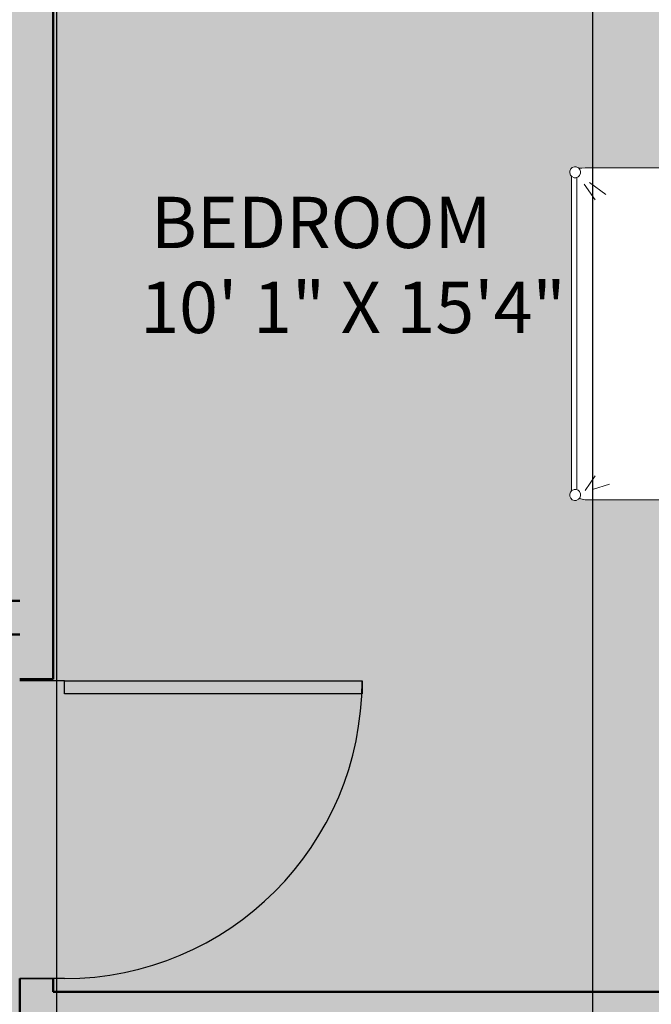
# Model space of a CAD drawing. Units: inches. Extents: x 528 to 2620, y -1066 to 798.
# Tile 32 of 41: x 1211 to 1296, y 524 to 656. Entities that reach past the tile are written whole.
import ezdxf

# ---------------------------------------------------------------- set-up
doc = ezdxf.new("R2010")
doc.units = ezdxf.units.IN
doc.header["$MEASUREMENT"] = 0
for name, color, linetype, lineweight in [('A-ANNO-DIMS', 2, 'Continuous', 18), ('A-AREA-IDEN', 7, 'Continuous', 18), ('A-Door', 2, 'Continuous', 25), ('A-FURN', 30, 'Continuous', 18), ('A-WALL', 7, 'Continuous', 50), ('A-WALL-PATT', 8, 'Continuous', 13)]:
    doc.layers.add(name, color=color, linetype=linetype, lineweight=lineweight)
doc.styles.get("Standard").update_dxf_attribs({"font": 'arial.ttf'})
doc.dimstyles.get("Standard").update_dxf_attribs({"dimtxt": 6, "dimasz": 2, "dimexe": 0.18, "dimexo": 0.0625, "dimgap": 0.09, "dimtad": 0, "dimtih": 1, "dimtoh": 1, "dimdec": 1, "dimzin": 0, "dimdsep": 46, "dimlunit": 3, "dimtxsty": 'Standard', "dimblk": 'ARCHTICK', "dimcen": 0.09, "dimadec": 0, "dimazin": 0, "dimtfac": 1, "dimtdec": 1, "dimtofl": 0, "dimtmove": 0, "dimatfit": 3, "dimfxl": 1, "dimtolj": 1, "dimtzin": 0, "dimarcsym": 0})

# ---------------------------------------------------------------- blocks, each defined once
blk = doc.blocks.new('*U4')
for p, q in [((0, 0), (0, -6)), ((40, 0), (40, -6))]:
    blk.add_line(p, q)
blk.add_lwpolyline([(0, 0), (0, 40), (1.75, 40), (1.75, 0)], close=True)
blk.add_arc((0, 0), 40, 0, 90)
blk = doc.blocks.new('d-bed-3')
at = {"color": 0, "linetype": 'ByBlock'}
for p, q in [((0, 0), (0, -0.5)), ((0.7, 0), (0, 0)), ((0.7, -0.5), (0.7, 0)), ((0.7817, -0.0054), (0.7857, 0.0078)), ((0.7817, -0.0054), (0.7857, 0.0078)), ((0.7857, 0.0078), (0.7968, 0.0166)), ((0.7857, 0.0078), (0.7968, 0.0166)), ((0.7968, 0.0166), (0.8078, 0.0211)), ((0.7968, 0.0166), (0.8078, 0.0211)), ((0.8078, 0.0211), (0.8209, 0.0211)), ((0.8078, 0.0211), (0.8209, 0.0211)), ((0.8209, 0.0211), (0.8349, 0.0144)), ((0.8209, 0.0211), (0.8349, 0.0144)), ((0.8349, 0.0144), (0.8409, 0.0078)), ((0.8349, 0.0144), (0.8429, 0.0056)), ((0.8389, 0.0078), (2.7305, 0.0078)), ((0.8409, 0.0078), (2.7305, 0.0078)), ((0.8429, 0.0056), (0.848, -0.0077)), ((2.7234, -0.0077), (2.7284, 0.0056)), ((2.7284, 0.0056), (2.7365, 0.0144)), ((2.7305, 0.0078), (2.7365, 0.0144)), ((2.7365, 0.0144), (2.7505, 0.0211)), ((2.7365, 0.0144), (2.7505, 0.0211)), ((2.7505, 0.0211), (2.7636, 0.0211)), ((2.7505, 0.0211), (2.7636, 0.0211)), ((2.7636, 0.0211), (2.7746, 0.0166)), ((2.7636, 0.0211), (2.7746, 0.0166)), ((2.7746, 0.0166), (2.7857, 0.0078)), ((2.7746, 0.0166), (2.7857, 0.0078)), ((2.7857, 0.0078), (2.7897, -0.0054)), ((2.7857, 0.0078), (2.7897, -0.0054)), ((2.8714, -0.5), (2.8714, 0)), ((2.8714, 0), (3.5714, 0)), ((3.5714, 0), (3.5714, -0.5)), ((0.05, -0.05), (0.05, -0.45)), ((0.65, -0.05), (0.05, -0.05)), ((0.35, -0.0576), (0.35, -0.4424)), ((0.65, -0.45), (0.65, -0.05)), ((0.7817, -0.0187), (0.7817, -0.0054)), ((0.7817, -0.0187), (0.7817, -0.0054)), ((0.7857, -0.0297), (0.7817, -0.0187)), ((0.7857, -0.0297), (0.7817, -0.0187)), ((0.7857, -2.0939), (0.7857, -0.0297)), ((0.7948, -0.0408), (0.7857, -0.0297)), ((0.7857, -0.032), (0.7857, -2.0939)), ((0.8058, -0.0452), (0.7948, -0.0408)), ((0.8188, -0.0452), (0.8058, -0.0452)), ((0.8319, -0.0408), (0.8188, -0.0452)), ((2.7525, -0.0452), (0.8188, -0.0452)), ((0.8409, -0.032), (0.8319, -0.0408)), ((0.848, -0.0209), (0.8409, -0.032)), ((0.848, -0.0077), (0.848, -0.0209)), ((2.7234, -0.0209), (2.7234, -0.0077)), ((2.7305, -0.032), (2.7234, -0.0209)), ((2.7395, -0.0408), (2.7305, -0.032)), ((2.7525, -0.0452), (2.7395, -0.0408)), ((2.7656, -0.0452), (2.7525, -0.0452)), ((2.7766, -0.0408), (2.7656, -0.0452)), ((2.7766, -0.0408), (2.7656, -0.0452)), ((2.7656, -0.0452), (2.7857, -0.0452)), ((2.7857, -0.0452), (2.7656, -0.0452)), ((2.7857, -0.0297), (2.7766, -0.0408)), ((2.7857, -0.0297), (2.7766, -0.0408)), ((2.7897, -0.0187), (2.7857, -0.0297)), ((2.7897, -0.0187), (2.7857, -0.0297)), ((2.7857, -2.0939), (2.7857, -0.0452)), ((2.7897, -0.0054), (2.7897, -0.0187)), ((2.7897, -0.0054), (2.7897, -0.0187)), ((2.9214, -0.45), (2.9214, -0.05)), ((2.9214, -0.05), (3.5214, -0.05)), ((3.2214, -0.0576), (3.2214, -0.4424)), ((3.5214, -0.05), (3.5214, -0.45)), ((0.8781, -0.1325), (0.8911, -0.1059)), ((0.8911, -0.1059), (0.9182, -0.1082)), ((0.9182, -0.1082), (0.9443, -0.1148)), ((0.9443, -0.1148), (0.9684, -0.128)), ((1.0056, -0.128), (1.0317, -0.117)), ((1.0317, -0.117), (1.0588, -0.1082)), ((1.0588, -0.1082), (1.0849, -0.1059)), ((1.0849, -0.1059), (1.113, -0.1104)), ((1.113, -0.1104), (1.1401, -0.117)), ((1.1401, -0.117), (1.1662, -0.128)), ((1.2034, -0.128), (1.2295, -0.117)), ((1.2295, -0.117), (1.2566, -0.1082)), ((1.2566, -0.1082), (1.2827, -0.1059)), ((1.2827, -0.1059), (1.3108, -0.1104)), ((1.3108, -0.1104), (1.3379, -0.117)), ((1.3379, -0.117), (1.362, -0.128)), ((1.4012, -0.128), (1.4253, -0.117)), ((1.4253, -0.117), (1.4514, -0.1082)), ((1.4514, -0.1082), (1.4805, -0.1059)), ((1.4805, -0.1059), (1.5086, -0.1104)), ((1.5086, -0.1104), (1.5357, -0.117)), ((1.5357, -0.117), (1.5598, -0.128)), ((1.5989, -0.128), (1.623, -0.1148)), ((1.623, -0.1148), (1.6471, -0.1082)), ((1.6471, -0.1082), (1.6763, -0.1059)), ((1.6763, -0.1059), (1.7084, -0.1059)), ((1.7084, -0.1059), (1.7194, -0.1325)), ((1.8489, -0.1302), (1.863, -0.1059)), ((1.863, -0.1059), (1.8951, -0.1059)), ((1.8951, -0.1059), (1.9222, -0.1059)), ((1.9222, -0.1059), (1.9483, -0.1148)), ((1.9483, -0.1148), (1.9724, -0.128)), ((2.0096, -0.128), (2.0357, -0.1148)), ((2.0357, -0.1148), (2.0628, -0.1082)), ((2.0628, -0.1082), (2.0909, -0.1059)), ((2.0909, -0.1059), (2.117, -0.1082)), ((2.117, -0.1082), (2.1441, -0.1148)), ((2.1441, -0.1148), (2.1702, -0.128)), ((2.2074, -0.128), (2.2335, -0.1148)), ((2.2335, -0.1148), (2.2606, -0.1082)), ((2.2606, -0.1082), (2.2867, -0.1059)), ((2.2867, -0.1059), (2.3148, -0.1082)), ((2.3148, -0.1082), (2.3419, -0.1148)), ((2.3419, -0.1148), (2.366, -0.128)), ((2.4052, -0.128), (2.4293, -0.1148)), ((2.4293, -0.1148), (2.4554, -0.1082)), ((2.4554, -0.1082), (2.4845, -0.1059)), ((2.4845, -0.1059), (2.5126, -0.1082)), ((2.5126, -0.1082), (2.5397, -0.1148)), ((2.5397, -0.1148), (2.5638, -0.128)), ((2.6029, -0.128), (2.627, -0.1148)), ((2.627, -0.1148), (2.6511, -0.1059)), ((2.6511, -0.1059), (2.6803, -0.1059)), ((2.6803, -0.1059), (2.6913, -0.1302)), ((0.8721, -0.159), (0.8781, -0.1325)), ((0.8741, -0.1866), (0.8721, -0.159)), ((0.9072, -0.5753), (0.9072, -0.1391)), ((0.9072, -0.1391), (1.6763, -0.1391)), ((0.9223, -0.1612), (0.9333, -0.2042)), ((0.9293, -0.1435), (0.9775, -0.1612)), ((0.9684, -0.128), (1.0056, -0.128)), ((1.1662, -0.128), (1.2034, -0.128)), ((1.362, -0.128), (1.4012, -0.128)), ((1.5598, -0.128), (1.5989, -0.128)), ((1.6471, -0.1501), (1.5989, -0.1656)), ((1.6542, -0.1656), (1.6431, -0.2087)), ((1.6763, -0.1391), (1.6763, -0.4936)), ((1.7194, -0.1325), (1.7265, -0.159)), ((1.7265, -0.159), (1.7265, -0.1866)), ((1.8429, -0.159), (1.8489, -0.1302)), ((1.8449, -0.1866), (1.8429, -0.159)), ((2.6622, -0.1369), (1.8931, -0.1369)), ((1.8931, -0.1369), (1.8931, -0.5046)), ((1.9152, -0.1656), (1.9263, -0.2087)), ((1.9222, -0.1479), (1.9704, -0.1656)), ((1.9724, -0.128), (2.0096, -0.128)), ((2.1702, -0.128), (2.2074, -0.128)), ((2.366, -0.128), (2.4052, -0.128)), ((2.5638, -0.128), (2.6029, -0.128)), ((2.6401, -0.1435), (2.5919, -0.159)), ((2.6471, -0.159), (2.6361, -0.202)), ((2.6622, -0.5753), (2.6622, -0.1369)), ((2.6913, -0.1302), (2.6973, -0.159)), ((2.6973, -0.159), (2.6973, -0.1866)), ((0.8831, -0.2131), (0.8741, -0.1866)), ((0.8962, -0.2374), (0.8831, -0.2131)), ((1.7174, -0.2131), (1.7024, -0.2374)), ((1.7265, -0.1866), (1.7174, -0.2131)), ((1.854, -0.2131), (1.8449, -0.1866)), ((1.867, -0.2374), (1.854, -0.2131)), ((2.6883, -0.2131), (2.6732, -0.2374)), ((2.6973, -0.1866), (2.6883, -0.2131)), ((0.1576, -0.25), (0.5424, -0.25)), ((0.8962, -0.2992), (0.8962, -0.2374)), ((1.7024, -0.2374), (1.7024, -0.2992)), ((1.867, -0.297), (1.867, -0.2374)), ((2.6732, -0.2374), (2.6732, -0.297)), ((3.4138, -0.25), (3.029, -0.25)), ((0.8761, -0.3489), (0.8831, -0.3235)), ((0.8761, -0.3776), (0.8761, -0.3489)), ((0.8831, -0.3235), (0.8962, -0.2992)), ((1.0538, -0.6294), (1.362, -0.3081)), ((1.3289, -0.3511), (1.3068, -0.3909)), ((1.362, -0.3081), (1.619, -0.5532)), ((1.4052, -0.3467), (1.4122, -0.4019)), ((1.7024, -0.2992), (1.7174, -0.3235)), ((1.7174, -0.3235), (1.7244, -0.3489)), ((1.7244, -0.3489), (1.7244, -0.3776)), ((1.8469, -0.3489), (1.854, -0.3213)), ((1.8469, -0.3754), (1.8469, -0.3489)), ((1.854, -0.3213), (1.867, -0.297)), ((2.2074, -0.3081), (1.9483, -0.5532)), ((2.1632, -0.3445), (2.1572, -0.3997)), ((2.5146, -0.6294), (2.2074, -0.3081)), ((2.2405, -0.3511), (2.2626, -0.3887)), ((2.6732, -0.297), (2.6883, -0.3213)), ((2.6883, -0.3213), (2.6953, -0.3489)), ((2.6953, -0.3489), (2.6953, -0.3754)), ((0.8831, -0.4041), (0.8761, -0.3776)), ((0.8962, -0.4284), (0.8831, -0.4041)), ((1.3068, -0.3909), (1.3349, -0.4174)), ((1.4122, -0.4019), (1.3901, -0.4284)), ((1.4674, -0.7134), (1.7746, -0.3909)), ((1.7174, -0.4041), (1.7024, -0.4284)), ((1.7244, -0.3776), (1.7174, -0.4041)), ((1.7746, -0.3909), (2.0979, -0.6979)), ((1.854, -0.4041), (1.8469, -0.3754)), ((1.867, -0.4284), (1.854, -0.4041)), ((2.1572, -0.3997), (2.1793, -0.4284)), ((2.2626, -0.3887), (2.2335, -0.4174)), ((2.6883, -0.4041), (2.6732, -0.4284)), ((2.6953, -0.3754), (2.6883, -0.4041)), ((0.05, -0.45), (0.65, -0.45)), ((0.8962, -0.4781), (0.8962, -0.4284)), ((1.2255, -0.4715), (1.2626, -0.5223)), ((1.5006, -0.4505), (1.4604, -0.4715)), ((1.5327, -0.4715), (1.4674, -0.5267)), ((1.7024, -0.4284), (1.7024, -0.4649)), ((1.7415, -0.4351), (1.7194, -0.4737)), ((1.7194, -0.4737), (1.7485, -0.5002)), ((1.8188, -0.4306), (1.8228, -0.4848)), ((1.867, -0.4781), (1.867, -0.4284)), ((2.0357, -0.4715), (2.102, -0.5267)), ((2.0688, -0.4505), (2.109, -0.4715)), ((2.3439, -0.4715), (2.3068, -0.5201)), ((2.6732, -0.4284), (2.6732, -0.4759)), ((3.5214, -0.45), (2.9214, -0.45)), ((0, -0.5), (0.7, -0.5)), ((0.8721, -0.5576), (0.8741, -0.5289)), ((0.8741, -0.5289), (0.8831, -0.5024)), ((0.8831, -0.5024), (0.8962, -0.4781)), ((0.9223, -0.5532), (0.9333, -0.5113)), ((1.8228, -0.4848), (1.8008, -0.5113)), ((1.9112, -0.5333), (1.874, -0.5554)), ((2.6471, -0.5532), (2.6361, -0.5091)), ((2.6732, -0.4759), (2.6883, -0.5002)), ((2.6883, -0.5002), (2.6973, -0.5267)), ((2.6973, -0.5267), (2.6973, -0.5554)), ((3.5714, -0.5), (2.8714, -0.5)), ((0.8781, -0.5841), (0.8721, -0.5576)), ((0.8911, -0.6096), (0.8781, -0.5841)), ((1.109, -0.5753), (0.9072, -0.5753)), ((0.9293, -0.5709), (0.9775, -0.5532)), ((0.9684, -0.5886), (0.9443, -0.6007)), ((1.0056, -0.5886), (0.9684, -0.5886)), ((1.0317, -0.5996), (1.0056, -0.5886)), ((1.105, -0.5864), (1.1271, -0.5864)), ((1.1271, -0.5864), (1.1482, -0.5974)), ((1.1482, -0.5974), (1.1311, -0.5864)), ((1.1311, -0.5864), (1.1592, -0.593)), ((1.2957, -0.5819), (1.2737, -0.5488)), ((1.3459, -0.625), (1.2957, -0.5819)), ((1.3399, -0.5643), (1.3399, -0.5488)), ((1.357, -0.625), (1.3399, -0.5643)), ((1.5658, -0.5753), (1.5377, -0.5864)), ((1.5969, -0.5753), (1.5658, -0.5753)), ((1.5989, -0.5488), (1.614, -0.5554)), ((1.6381, -0.5554), (1.6763, -0.6051)), ((1.9443, -0.5554), (1.8781, -0.6096)), ((1.9704, -0.5466), (1.9503, -0.5554)), ((1.9684, -0.5753), (2.0036, -0.5753)), ((2.0036, -0.5753), (2.0317, -0.5864)), ((2.2124, -0.6228), (2.2295, -0.5643)), ((2.2224, -0.6228), (2.2736, -0.5797)), ((2.2295, -0.5643), (2.2295, -0.5466)), ((2.2736, -0.5797), (2.2957, -0.5466)), ((2.4383, -0.5864), (2.4092, -0.5908)), ((2.4423, -0.5864), (2.4202, -0.5974)), ((2.4202, -0.5974), (2.4383, -0.5864)), ((2.4644, -0.5864), (2.4423, -0.5864)), ((2.4604, -0.5753), (2.6622, -0.5753)), ((2.5638, -0.5864), (2.5397, -0.5996)), ((2.6029, -0.5864), (2.5638, -0.5864)), ((2.6401, -0.5687), (2.5919, -0.5532)), ((2.627, -0.5996), (2.6029, -0.5864)), ((2.6913, -0.5841), (2.6803, -0.6073)), ((2.6973, -0.5554), (2.6913, -0.5841)), ((0.9182, -0.6073), (0.8911, -0.6096)), ((0.9443, -0.6007), (0.9182, -0.6073)), ((1.0588, -0.6073), (1.0317, -0.5996)), ((1.3791, -0.9365), (1.0538, -0.6294)), ((1.0759, -0.6096), (1.0588, -0.6073)), ((1.3138, -0.6626), (1.351, -0.6361)), ((1.368, -0.6626), (1.357, -0.625)), ((1.3731, -0.6294), (1.4453, -0.614)), ((1.3791, -0.6471), (1.4453, -0.6913)), ((1.7084, -0.6648), (1.6873, -0.6316)), ((1.7526, -0.6493), (1.7526, -0.6316)), ((1.7706, -0.7089), (1.7526, -0.6493)), ((2.0387, -0.6427), (2.0427, -0.6405)), ((2.1963, -0.6294), (2.124, -0.6118)), ((2.1903, -0.6449), (2.124, -0.6891)), ((2.1903, -0.9365), (2.5146, -0.6294)), ((2.2013, -0.6626), (2.2124, -0.6228)), ((2.2556, -0.6626), (2.2184, -0.6338)), ((2.5126, -0.6051), (2.4955, -0.6073)), ((2.5397, -0.5996), (2.5126, -0.6051)), ((2.6511, -0.6073), (2.627, -0.5996)), ((2.6803, -0.6073), (2.6511, -0.6073)), ((1.105, -0.6692), (1.1421, -0.6846)), ((1.1421, -0.6846), (1.1642, -0.6736)), ((1.1642, -0.6736), (1.1753, -0.6692)), ((1.3731, -0.6692), (1.3841, -0.7067)), ((1.4674, -0.7134), (1.4604, -0.7067)), ((1.7596, -0.7089), (1.7084, -0.6648)), ((1.7817, -0.7454), (1.7706, -0.7089)), ((1.7857, -0.7134), (1.856, -0.6979)), ((2.0979, -0.6979), (1.7897, -1.0193)), ((1.9765, -0.6604), (1.9503, -0.6714)), ((2.0166, -0.6604), (1.9765, -0.6604)), ((2.0387, -0.6714), (2.0166, -0.6604)), ((2.0538, -0.7609), (2.109, -0.7067)), ((2.1963, -0.667), (2.1853, -0.7067)), ((2.4052, -0.6736), (2.3941, -0.667)), ((2.4272, -0.6846), (2.4052, -0.6736)), ((2.4644, -0.667), (2.4272, -0.6846)), ((1.2255, -0.7785), (1.2737, -0.7244)), ((1.7897, -1.0193), (1.4674, -0.7134)), ((1.5548, -0.7675), (1.5397, -0.7631)), ((1.5548, -0.7675), (1.5769, -0.7564)), ((1.5769, -0.7564), (1.5879, -0.752)), ((1.7265, -0.7454), (1.7636, -0.72)), ((1.7857, -0.752), (1.7967, -0.7896)), ((1.7897, -0.731), (1.856, -0.7741)), ((1.9724, -0.741), (1.9393, -0.7244)), ((2.0096, -0.741), (1.9724, -0.741)), ((2.0497, -0.731), (2.0096, -0.741)), ((2.1903, -0.9365), (2.0277, -0.7697)), ((2.3439, -0.7763), (2.2957, -0.7222)), ((0.7857, -0.9607), (1.2295, -0.8072)), ((0.9504, -1.2611), (1.5708, -0.8183)), ((1.3178, -0.8382), (1.3239, -0.8117)), ((1.3791, -0.9365), (1.5357, -0.7763)), ((1.6381, -0.8625), (1.6873, -0.8072)), ((1.9283, -0.8448), (1.874, -0.7896)), ((2.618, -1.2611), (1.9855, -0.8161)), ((2.2515, -0.8382), (2.2445, -0.8094)), ((2.7827, -0.9607), (2.3278, -0.8072)), ((1.3178, -0.8602), (1.3178, -0.8382)), ((1.3349, -0.8879), (1.3178, -0.8602)), ((1.3901, -0.8989), (1.4052, -0.8768)), ((1.4052, -0.8337), (1.4012, -0.8337)), ((1.4052, -0.8768), (1.4052, -0.8337)), ((2.1632, -0.8757), (2.1632, -0.8315)), ((2.1632, -0.8315), (2.1682, -0.8315)), ((2.1793, -0.8967), (2.1632, -0.8757)), ((2.2335, -0.8856), (2.2515, -0.8602)), ((2.2515, -0.8602), (2.2515, -0.8382)), ((0.8781, -1.2059), (1.3349, -0.9055)), ((1.7305, -0.921), (1.7375, -0.8945)), ((1.7305, -0.9431), (1.7305, -0.921)), ((1.7485, -0.9718), (1.7305, -0.9431)), ((1.8188, -0.9166), (1.8118, -0.9166)), ((1.8188, -0.9607), (1.8188, -0.9166)), ((2.6913, -1.2059), (2.2254, -0.9055)), ((0.8128, -1.0115), (0.7857, -0.9607)), ((1.8008, -0.9828), (1.8188, -0.9607)), ((2.7676, -0.9895), (2.7455, -1.0259)), ((2.7786, -0.9828), (2.7676, -0.9895)), ((2.7827, -0.9607), (2.7786, -0.9828)), ((0.8128, -1.0325), (0.8128, -1.0115)), ((0.8239, -1.0414), (0.8128, -1.0325)), ((0.8299, -1.0635), (0.8239, -1.0414)), ((0.8349, -1.0745), (0.8299, -1.0635)), ((2.7455, -1.0259), (2.7234, -1.0811)), ((0.845, -1.1032), (0.8349, -1.0745)), ((0.852, -1.1187), (0.845, -1.1032)), ((0.852, -1.1363), (0.852, -1.1187)), ((2.7124, -1.1253), (2.6953, -1.1617)), ((2.7174, -1.1187), (2.7124, -1.1253)), ((2.7234, -1.1076), (2.7174, -1.1187)), ((2.7234, -1.0811), (2.7234, -1.1076)), ((0.863, -1.1617), (0.852, -1.1363)), ((0.867, -1.1905), (0.863, -1.1617)), ((0.9223, -1.2015), (0.9112, -1.1838)), ((2.6582, -1.1838), (2.6471, -1.2015)), ((2.6953, -1.1617), (2.6913, -1.2059)), ((0.8741, -1.1949), (0.867, -1.1905)), ((0.8781, -1.2059), (0.8741, -1.1949)), ((0.9293, -1.2059), (0.9223, -1.2015)), ((0.9403, -1.2236), (0.9293, -1.2059)), ((0.9443, -1.2391), (0.9403, -1.2236)), ((0.9504, -1.2611), (0.9443, -1.2391)), ((2.625, -1.2391), (2.618, -1.2611)), ((2.6361, -1.2236), (2.625, -1.2391)), ((2.6471, -1.2015), (2.6361, -1.2236)), ((2.7234, -2.0497), (2.6913, -1.947)), ((0.8741, -2.0673), (0.9464, -1.9691)), ((0.8851, -2.1005), (0.9795, -2.0342)), ((2.7305, -2.0939), (2.6421, -2.0342)), ((0.7797, -2.148), (0.7857, -2.1347)), ((0.7797, -2.148), (0.7857, -2.1347)), ((0.7888, -2.1317), (0.7857, -2.0939)), ((0.7857, -2.0939), (0.7887, -2.1303)), ((0.7857, -2.1347), (0.7948, -2.1259)), ((0.7857, -2.1347), (0.7888, -2.1317)), ((0.7948, -2.1259), (0.8078, -2.1215)), ((0.8078, -2.1215), (0.8188, -2.1215)), ((0.8188, -2.1215), (0.8319, -2.1281)), ((0.8319, -2.1281), (0.8409, -2.1369)), ((2.7365, -2.1281), (2.7284, -2.1369)), ((2.7505, -2.1215), (2.7365, -2.1281)), ((2.7616, -2.1215), (2.7505, -2.1215)), ((2.7746, -2.1259), (2.7616, -2.1215)), ((2.7827, -2.1347), (2.7746, -2.1259)), ((2.7857, -2.0939), (2.7783, -2.1299)), ((2.7783, -2.1299), (2.7827, -2.1347)), ((2.7786, -2.1281), (2.7857, -2.0939)), ((2.7827, -2.1347), (2.7897, -2.148)), ((2.7897, -2.148), (2.7827, -2.1347)), ((0.7797, -2.159), (0.7797, -2.148)), ((0.7797, -2.148), (0.7797, -2.159)), ((0.7837, -2.1723), (0.7797, -2.159)), ((0.7837, -2.1723), (0.7797, -2.159)), ((0.7927, -2.1811), (0.7837, -2.1723)), ((0.7927, -2.1811), (0.7837, -2.1723)), ((0.8058, -2.1877), (0.7927, -2.1811)), ((0.8058, -2.1877), (0.7927, -2.1811)), ((0.8168, -2.1877), (0.8058, -2.1877)), ((0.8168, -2.1877), (0.8058, -2.1877)), ((0.8299, -2.1833), (0.8168, -2.1877)), ((0.8299, -2.1833), (0.8168, -2.1877)), ((0.8389, -2.1745), (0.8299, -2.1833)), ((0.8367, -2.1767), (0.8299, -2.1833)), ((2.7327, -2.1767), (0.8367, -2.1767)), ((0.845, -2.1612), (0.8389, -2.1745)), ((0.8389, -2.1767), (2.7305, -2.1767)), ((0.8409, -2.1369), (0.845, -2.1502)), ((2.7264, -2.1436), (0.845, -2.1436)), ((0.845, -2.1502), (0.845, -2.1612)), ((2.7284, -2.1369), (2.7234, -2.1502)), ((2.7234, -2.1502), (2.7234, -2.1612)), ((2.7234, -2.1612), (2.7305, -2.1745)), ((2.7305, -2.1745), (2.7395, -2.1833)), ((2.7395, -2.1833), (2.7327, -2.1767)), ((2.7525, -2.1877), (2.7395, -2.1833)), ((2.7395, -2.1833), (2.7525, -2.1877)), ((2.7636, -2.1877), (2.7525, -2.1877)), ((2.7525, -2.1877), (2.7636, -2.1877)), ((2.7766, -2.1811), (2.7636, -2.1877)), ((2.7636, -2.1877), (2.7766, -2.1811)), ((2.7857, -2.1723), (2.7766, -2.1811)), ((2.7766, -2.1811), (2.7857, -2.1723)), ((2.7897, -2.159), (2.7857, -2.1723)), ((2.7857, -2.1723), (2.7897, -2.159)), ((2.7897, -2.148), (2.7897, -2.159)), ((2.7897, -2.159), (2.7897, -2.148))]:
    blk.add_line(p, q, dxfattribs=at)
blk.add_ellipse((0.35, -0.25), major_axis=(-0.1007, 0.1007), ratio=1, dxfattribs=at)
at = {"color": 0, "linetype": 'ByBlock', "extrusion": (0, 0, -1)}
blk.add_ellipse((3.2214, -0.25), major_axis=(0.1007, 0.1007), ratio=1, dxfattribs=at)
blk = doc.blocks.new('_ArchTick')
at = {"color": 0, "linetype": 'ByBlock', "const_width": 0.15}
blk.add_lwpolyline([(-0.5, -0.5), (0.5, 0.5)], dxfattribs=at)
blk = doc.blocks.new('*D68')
at = {"layer": 'A-ANNO-DIMS', "color": 0, "lineweight": -2, "transparency": 16777216}
for p, q in [((1216, 400.48), (1216, 751.1)), ((1216, 750.92), (1243.92, 750.92)), ((1288, 750.92), (1260.08, 750.92)), ((1288, 395.98), (1288, 751.1))]:
    blk.add_line(p, q, dxfattribs=at)
at = {"layer": 'Defpoints', "color": 0, "transparency": 16777216}
for p in [(1288, 750.92), (1216, 400.42), (1288, 395.92)]:
    blk.add_point(p, dxfattribs=at)
at = {"layer": 'A-ANNO-DIMS', "color": 0, "lineweight": -2, "transparency": 16777216, "xscale": 2, "yscale": 2, "zscale": 2, "rotation": 180}
blk.add_blockref('_ArchTick', (1216, 750.92), dxfattribs=at)
at = {"layer": 'A-ANNO-DIMS', "color": 0, "lineweight": -2, "transparency": 16777216, "xscale": 2, "yscale": 2, "zscale": 2}
blk.add_blockref('_ArchTick', (1288, 750.92), dxfattribs=at)
at = {"layer": 'A-ANNO-DIMS', "color": 0, "transparency": 16777216, "insert": (1252, 750.92), "char_height": 6, "attachment_point": 5}
blk.add_mtext('\\A1;6\'-0"', dxfattribs=at)

msp = doc.modelspace()

# ---------------------------------------------------------------- hatches: boundary and pattern name
at = {"layer": 'A-WALL-PATT', "transparency": 33554521}
h = msp.add_hatch(color=256, dxfattribs=at)
h.dxf.hatch_style = 1
h.paths.add_polyline_path([(1066, 709.92), (1114.5, 709.92), (1114.5, 718.92), (1057, 718.92), (1057, 667.92), (1066, 667.92)])
h.paths.add_polyline_path([(1227.5, 718.92), (1162.5, 718.92), (1162.5, 709.92), (1211, 709.92), (1211, 577.92), (1205.42, 577.92), (1205.5, 573.42), (1211, 573.42), (1211, 567.42), (1215.5, 567.42), (1215.5, 669.42), (1268, 669.42), (1268, 675.92), (1263.5, 675.92), (1263.5, 673.92), (1215.5, 673.92), (1215.5, 709.92), (1227.5, 709.92)])
h.paths.add_polyline_path([(1345, 718.92), (1316, 718.92), (1316, 709.92), (1336, 709.92), (1336, 641.67), (1345, 641.67)])
h.paths.add_polyline_path([(1066, 619.92), (1057, 619.92), (1057, 561.42), (1066, 561.42), (1066, 573.42), (1161, 573.42), (1161, 569.42), (1165.5, 569.42), (1165.5, 577.92), (1066, 577.92)])
h.paths.add_polyline_path([(1216, 391.42), (1216, 400.42), (1207, 400.42), (1201, 400.42), (1201, 397.42), (1201, 391.42), (1207, 391.42), (1207, 268.92), (1252, 268.92), (1252, 277.92), (1216, 277.92), (1216, 359.77)])
h.paths.add_polyline_path([(1345, 395.92), (1336, 395.92), (1288, 395.92), (1288, 391.42), (1336, 391.42), (1336, 277.92), (1300, 277.92), (1300, 268.92), (1345, 268.92)])
h.paths.add_polyline_path([(1345, 593.67), (1336, 593.67), (1336, 525.42), (1215.5, 525.42), (1215.5, 527.17), (1211, 527.17), (1211, 520.92), (1336, 520.92), (1336, 443.92), (1345, 443.92)])
h.paths.add_polyline_path([(1066, 520.92), (1165.5, 520.92), (1165.5, 545.42), (1161, 545.42), (1161, 525.42), (1066, 525.42), (1066, 537.42), (1057, 537.42), (1057, 484.67), (1066, 484.67)])
h.paths.add_polyline_path([(1066, 436.67), (1057, 436.67), (1057, 391.42), (1085.5, 391.42), (1085.5, 400.42), (1066, 400.42)])
h.paths.add_polyline_path([(1153, 397.42), (1153, 400.42), (1133.5, 400.42), (1133.5, 391.42), (1153, 391.42)])
at = {"layer": 'A-WALL-PATT', "transparency": 33554536}
h = msp.add_hatch(color=256, dxfattribs=at)
h.dxf.hatch_style = 1
h.paths.add_polyline_path([(1336, 709.92), (1268, 709.92), (1268, 699.92), (1266.75, 699.92), (1266.75, 675.92), (1268, 675.92), (1268, 669.42), (1215.5, 669.42), (1215.5, 567.17), (1217, 567.17), (1257, 567.17), (1257, 565.42), (1256.96, 565.42, -0.401453), (1217, 527.17), (1215.5, 527.17), (1215.5, 525.42), (1336, 525.42)], flags=17)
h.paths.add_polyline_path([(1285.03, 635.93), (1285.23, 636.13), (1285.67, 636.26), (1286.21, 636.02), (1286.98, 636.08), (1332.98, 636.08), (1333.36, 636.22), (1333.82, 636.08), (1334.11, 635.71), (1334.11, 635.3), (1333.91, 634.86), (1333.82, 634.83), (1333.82, 592.74), (1333.97, 592.6), (1334.11, 592.29), (1334.11, 591.88), (1333.82, 591.51), (1333.36, 591.37), (1332.98, 591.51), (1332.64, 591.79), (1332.64, 591.51), (1286.98, 591.51), (1286.17, 591.67), (1286.07, 591.57), (1285.68, 591.37), (1285.23, 591.51), (1285.03, 591.71), (1284.83, 592.1), (1284.98, 592.54), (1285.13, 592.69), (1285.13, 634.95), (1284.98, 635.1), (1284.83, 635.54)], flags=16)
h.paths.add_polyline_path([(1285.03, 635.93), (1285.23, 636.13), (1285.67, 636.26), (1286.21, 636.02), (1286.98, 636.08), (1332.98, 636.08), (1333.36, 636.22), (1333.82, 636.08), (1334.11, 635.71), (1334.11, 635.3), (1333.97, 634.99), (1333.82, 634.85), (1333.82, 592.74), (1333.97, 592.6), (1334.11, 592.29), (1334.11, 591.88), (1333.82, 591.51), (1333.36, 591.37), (1332.98, 591.51), (1332.64, 591.79), (1332.64, 592.25), (1332.64, 635.35), (1332.64, 635.8), (1332.98, 636.08), (1312.23, 636.08), (1311.1, 635.48), (1310.63, 635.48), (1310.43, 635.23), (1309.94, 635.1), (1309.7, 634.99), (1309.06, 634.76), (1308.71, 634.61), (1308.32, 634.61), (1307.75, 634.36), (1307.11, 634.27), (1307.01, 634.11), (1306.77, 634.02), (1307.25, 633.28), (1306.87, 633.04), (1306.77, 632.88), (1306.37, 632.64), (1306.03, 632.55), (1305.54, 632.41), (1315.47, 618.49), (1316.32, 619.39), (1312.77, 622.86), (1319.62, 630.11), (1320.07, 629.68), (1320.11, 630), (1320.28, 630.6), (1320.53, 631.18), (1320.53, 632.01), (1320.26, 632.55), (1320.11, 633.13), (1320.06, 633.73), (1320.63, 634.02), (1321.22, 634.16), (1321.86, 634.11), (1322.45, 633.91), (1322.99, 633.62), (1324.1, 633.62), (1324.64, 633.91), (1325.23, 634.07), (1325.87, 634.07), (1326.43, 633.91), (1326.98, 633.62), (1328.35, 633.62), (1328.9, 633.91), (1329.49, 634.11), (1330.1, 634.16), (1330.69, 634.02), (1331.28, 633.73), (1331.23, 633.13), (1331.09, 632.55), (1330.79, 632.01), (1330.79, 631.18), (1331.04, 630.6), (1331.23, 630), (1331.28, 629.41), (1331.19, 628.79), (1331.04, 628.18), (1330.79, 627.6), (1330.79, 626.77), (1331.04, 626.19), (1331.23, 625.59), (1331.28, 625.01), (1331.19, 624.38), (1331.04, 623.78), (1330.79, 623.24), (1330.79, 622.37), (1331.04, 621.83), (1331.23, 621.25), (1331.28, 620.6), (1331.19, 619.97), (1331.04, 619.37), (1330.79, 618.83), (1330.79, 617.96), (1331.09, 617.42), (1331.23, 616.88), (1331.28, 616.23), (1331.28, 615.52), (1330.69, 615.27), (1330.1, 615.12), (1329.49, 615.12), (1328.9, 615.32), (1328.35, 615.65), (1326.98, 615.65), (1326.43, 615.32), (1325.87, 615.16), (1325.23, 615.16), (1324.64, 615.32), (1324.1, 615.65), (1323.24, 615.65), (1324.93, 614.04), (1322.98, 611.98), (1324.1, 611.98), (1324.64, 612.27), (1325.28, 612.43), (1325.87, 612.43), (1326.48, 612.27), (1327.03, 611.98), (1328.35, 611.98), (1328.9, 612.27), (1329.49, 612.48), (1330.1, 612.52), (1330.74, 612.39), (1331.28, 612.07), (1331.28, 611.36), (1331.28, 610.75), (1331.09, 610.17), (1330.79, 609.63), (1330.79, 608.81), (1331.09, 608.22), (1331.23, 607.62), (1331.28, 606.99), (1331.23, 606.41), (1331.09, 605.81), (1330.79, 605.22), (1330.79, 604.4), (1331.09, 603.81), (1331.23, 603.21), (1331.28, 602.63), (1331.23, 602), (1331.09, 601.4), (1330.79, 600.86), (1330.79, 599.99), (1331.09, 599.45), (1331.23, 598.87), (1331.28, 598.22), (1331.23, 597.59), (1331.09, 596.99), (1330.79, 596.45), (1330.79, 595.58), (1331.09, 595.04), (1331.28, 594.51), (1331.28, 593.86), (1330.74, 593.61), (1330.1, 593.48), (1329.49, 593.48), (1328.9, 593.68), (1328.35, 594.01), (1327.03, 594.01), (1326.48, 593.68), (1325.87, 593.52), (1325.28, 593.52), (1324.64, 593.68), (1324.1, 594.01), (1323.04, 594.01), (1322.5, 593.68), (1321.91, 593.48), (1321.27, 593.48), (1320.63, 593.61), (1320.11, 593.86), (1320.11, 594.51), (1320.28, 595.04), (1320.58, 595.58), (1320.58, 596.45), (1320.28, 596.99), (1320.16, 597.59), (1320.1, 598.01), (1319.62, 597.55), (1315.66, 601.73), (1312.23, 591.57), (1311.74, 591.66), (1311.59, 591.91), (1310.78, 592.4), (1309.55, 592.89), (1308.96, 592.89), (1308.71, 593.03), (1308.56, 593.14), (1307.75, 593.52), (1306.77, 593.61), (1307.25, 594.36), (1306.87, 594.6), (1306.37, 594.84), (1306.03, 595.09), (1305.54, 595.24), (1315.46, 609.35), (1310.93, 613.71), (1315.47, 618.49), (1305.54, 632.41), (1306.03, 632.55), (1306.37, 632.64), (1306.77, 632.88), (1306.87, 633.04), (1307.25, 633.28), (1306.77, 634.02), (1307.01, 634.11), (1307.11, 634.27), (1307.75, 634.36), (1308.32, 634.61), (1308.71, 634.61), (1309.06, 634.76), (1309.7, 634.99), (1309.94, 635.1), (1310.43, 635.23), (1310.63, 635.48), (1311.1, 635.48), (1312.23, 636.08), (1286.98, 636.08), (1286.22, 636.02), (1286.41, 635.44), (1286.21, 635.05), (1286.02, 634.85), (1285.87, 634.81), (1285.87, 592.84), (1286.15, 592.73), (1286.41, 592.19), (1286.23, 591.66), (1286.17, 591.67), (1286.07, 591.57), (1285.68, 591.37), (1285.23, 591.51), (1285.03, 591.71), (1284.83, 592.1), (1284.98, 592.54), (1285.13, 592.69), (1285.13, 634.95), (1284.98, 635.1), (1284.83, 635.54)], flags=0)
h.paths.add_polyline_path([(1322.5, 653.6), (1333.65, 653.6), (1333.65, 637.99), (1322.5, 637.99)], flags=16)
h.paths.add_polyline_path([(1323.62, 652.48), (1332.53, 652.48), (1332.53, 639.11), (1323.62, 639.11)], flags=0)
edge = h.paths.add_edge_path(flags=0)
edge.add_ellipse((1328.07, 645.79), major_axis=(2.24, 2.24), ratio=1, start_angle=405, end_angle=495, ccw=False)
edge.add_ellipse((1328.07, 645.79), major_axis=(2.24, 2.24), ratio=1, start_angle=675, end_angle=765, ccw=False)
edge.add_ellipse((1328.07, 645.79), major_axis=(2.24, 2.24), ratio=1, start_angle=585, end_angle=675, ccw=False)
edge.add_ellipse((1328.07, 645.79), major_axis=(2.24, 2.24), ratio=1, start_angle=495, end_angle=585, ccw=False)
h.paths.add_polyline_path([(1320.58, 628.39), (1320.33, 628.01), (1320.61, 628.55)], flags=0)
h.paths.add_polyline_path([(1317.89, 604.89), (1318.78, 604.64), (1319.76, 604.28), (1318.88, 604.53)], flags=0)
h.paths.add_polyline_path([(1320.33, 599.65), (1320.58, 599.25), (1320.58, 599.16)], flags=0)
h.paths.add_polyline_path([(1322.5, 589.6), (1333.65, 589.6), (1333.65, 573.99), (1322.5, 573.99)], flags=16)
h.paths.add_polyline_path([(1323.62, 588.48), (1332.53, 588.48), (1332.53, 575.11), (1323.62, 575.11)], flags=0)
edge = h.paths.add_edge_path(flags=0)
edge.add_ellipse((1328.07, 581.8), major_axis=(-2.24, 2.24), ratio=1, start_angle=-45, end_angle=45, ccw=False)
edge.add_ellipse((1328.07, 581.8), major_axis=(-2.24, 2.24), ratio=1, start_angle=-135, end_angle=-45, ccw=False)
edge.add_ellipse((1328.07, 581.8), major_axis=(-2.24, 2.24), ratio=1, start_angle=135, end_angle=-135, ccw=False)
edge.add_ellipse((1328.07, 581.8), major_axis=(-2.24, 2.24), ratio=1, start_angle=45, end_angle=135, ccw=False)
h.paths.add_polyline_path([(1264.75, 699.92), (1263.5, 699.92), (1263.5, 709.92), (1215.5, 709.92), (1215.5, 673.92), (1263.5, 673.92), (1263.5, 675.92), (1264.75, 675.92)], flags=16)
h.paths.add_polyline_path([(1162.19, 569.42), (1161, 569.42), (1161, 573.42), (1066, 573.42), (1066, 525.42), (1161, 525.42), (1161, 545.42), (1162.19, 545.42)])
h.paths.add_polyline_path([(1256.96, 565.42), (1257, 565.42), (1257, 567.17), (1217, 567.17), (1215.5, 567.17), (1215.5, 567.42), (1211, 567.42), (1211, 573.42), (1205.5, 573.42), (1205.42, 577.92), (1211, 577.92), (1211, 709.92), (1066, 709.92), (1066, 577.92), (1165.5, 577.92), (1165.5, 569.42), (1164.19, 569.42), (1164.19, 545.42), (1165.5, 545.42), (1165.5, 520.92), (1153, 520.92), (1153, 484.92), (1102, 484.92), (1102, 436.42), (1153, 436.42), (1153, 400.42), (1153, 391.42), (1201, 391.42), (1201, 400.42), (1207, 400.42), (1216, 400.42), (1216, 391.42), (1216, 277.92), (1336, 277.92), (1336, 391.42), (1288, 391.42), (1288, 395.92), (1336, 395.92), (1336, 443.92), (1336, 520.92), (1211, 520.92), (1211, 527.17), (1215.5, 527.17), (1217, 527.17, 0.401453)])
h.paths.add_polyline_path([(1167.25, 579.42), (1165.5, 579.42), (1165.5, 619.42), (1167.25, 619.42)], flags=16)
h.paths.add_polyline_path([(1227.97, 501.56), (1236.36, 502.03), (1236.36, 492.55), (1227.97, 493.02, -0.254069)], flags=16)
h.paths.add_polyline_path([(1243.34, 515.69, -0.254069), (1251.88, 515.69), (1252.35, 507.3), (1242.87, 507.3)], flags=16)
h.paths.add_polyline_path([(1239.18, 504.68), (1256.03, 504.68), (1256.03, 479.42), (1239.18, 479.42)], flags=16)
h.paths.add_polyline_path([(1227.97, 489.6), (1236.36, 490.07), (1236.36, 480.59), (1227.97, 481.06, -0.254069)], flags=16)
h.paths.add_polyline_path([(1197.2, 624.04), (1197.2, 639.64), (1208.35, 639.64), (1208.35, 624.04)], flags=16)
h.paths.add_polyline_path([(1198.32, 625.15), (1198.32, 638.53), (1207.23, 638.53), (1207.23, 625.15)], flags=0)
h.paths.add_polyline_path([(1258.85, 502.03), (1267.25, 501.56, -0.254069), (1267.25, 493.02), (1258.85, 492.55)], flags=16)
h.paths.add_polyline_path([(1271.59, 519.66), (1333.67, 519.66), (1333.67, 451.59), (1319.09, 451.59), (1319.09, 505.07), (1288.09, 505.07), (1284.45, 505.07, -0.883215), (1270.68, 514.19), (1270.68, 518.75, -0.414214)], flags=16)
h.paths.add_polyline_path([(1331.85, 517.83), (1331.85, 453.42), (1328.2, 453.42), (1328.2, 505.07), (1298.42, 505.07), (1298.42, 514.19), (1288.09, 514.19), (1288.09, 517.83)], flags=0)
h.paths.add_polyline_path([(1242.87, 476.8), (1252.35, 476.8), (1251.88, 468.41, -0.254069), (1243.34, 468.41)], flags=16)
h.paths.add_polyline_path([(1258.85, 490.07), (1267.25, 489.6, -0.254069), (1267.25, 481.06), (1258.85, 480.59)], flags=16)
h.paths.add_polyline_path([(1161.68, 641.55), (1160.87, 641.72), (1160.77, 641.62), (1160.38, 641.41), (1159.93, 641.55), (1159.73, 641.75), (1159.53, 642.14), (1159.68, 642.58), (1159.83, 642.73), (1159.83, 684.99), (1159.68, 685.14), (1159.53, 685.58), (1159.73, 685.97), (1159.93, 686.17), (1160.37, 686.31), (1160.91, 686.06), (1161.68, 686.13), (1207.68, 686.13), (1208.06, 686.27), (1208.52, 686.13), (1208.81, 685.76), (1208.81, 685.34), (1208.61, 684.9), (1208.52, 684.87), (1208.52, 642.78), (1208.67, 642.65), (1208.88, 642.2), (1208.72, 641.8), (1208.52, 641.55), (1208.06, 641.41), (1207.68, 641.55), (1207.34, 641.83), (1207.34, 641.55)], flags=16)
h.paths.add_polyline_path([(1186.93, 641.62), (1186.44, 641.71), (1186.29, 641.95), (1185.48, 642.45), (1184.25, 642.94), (1183.66, 642.94), (1183.41, 643.07), (1183.26, 643.18), (1182.45, 643.57), (1181.47, 643.65), (1181.95, 644.4), (1181.57, 644.64), (1181.07, 644.89), (1180.73, 645.13), (1180.24, 645.29), (1190.16, 659.4), (1185.63, 663.75), (1190.17, 668.54), (1180.24, 682.46), (1180.73, 682.59), (1181.07, 682.68), (1181.47, 682.93), (1181.57, 683.08), (1181.95, 683.33), (1181.47, 684.07), (1181.71, 684.16), (1181.81, 684.31), (1182.45, 684.4), (1183.02, 684.65), (1183.41, 684.65), (1183.76, 684.81), (1184.4, 685.03), (1184.64, 685.14), (1185.13, 685.28), (1185.33, 685.52), (1185.8, 685.52), (1186.93, 686.13), (1161.68, 686.13), (1160.92, 686.06), (1161.11, 685.49), (1160.91, 685.1), (1160.72, 684.9), (1160.57, 684.85), (1160.57, 642.88), (1160.85, 642.77), (1161.11, 642.23), (1160.93, 641.7), (1160.87, 641.72), (1160.77, 641.62), (1160.38, 641.41), (1159.93, 641.55), (1159.73, 641.75), (1159.53, 642.14), (1159.68, 642.58), (1159.83, 642.73), (1159.83, 684.99), (1159.68, 685.14), (1159.53, 685.58), (1159.73, 685.97), (1159.93, 686.17), (1160.37, 686.31), (1160.91, 686.06), (1161.68, 686.13), (1207.68, 686.13), (1208.06, 686.27), (1208.52, 686.13), (1208.81, 685.76), (1208.81, 685.34), (1208.67, 685.03), (1208.52, 684.9), (1208.52, 642.78), (1208.67, 642.65), (1208.88, 642.2), (1208.72, 641.8), (1208.52, 641.55), (1208.06, 641.41), (1207.68, 641.55), (1207.34, 641.83), (1207.34, 642.29), (1207.34, 685.39), (1207.34, 685.85), (1207.68, 686.13), (1186.93, 686.13), (1185.8, 685.52), (1185.33, 685.52), (1185.13, 685.28), (1184.64, 685.14), (1184.4, 685.03), (1183.76, 684.81), (1183.41, 684.65), (1183.02, 684.65), (1182.45, 684.4), (1181.81, 684.31), (1181.71, 684.16), (1181.47, 684.07), (1181.95, 683.33), (1181.57, 683.08), (1181.47, 682.93), (1181.07, 682.68), (1180.73, 682.59), (1180.24, 682.46), (1190.17, 668.54), (1191.02, 669.43), (1187.47, 672.9), (1194.32, 680.15), (1194.77, 679.72), (1194.81, 680.04), (1194.98, 680.65), (1195.23, 681.23), (1195.23, 682.05), (1194.96, 682.59), (1194.81, 683.17), (1194.76, 683.78), (1195.33, 684.07), (1195.92, 684.2), (1196.56, 684.16), (1197.15, 683.96), (1197.69, 683.67), (1198.8, 683.67), (1199.34, 683.96), (1199.93, 684.11), (1200.57, 684.11), (1201.13, 683.96), (1201.68, 683.67), (1203.05, 683.67), (1203.6, 683.96), (1204.19, 684.16), (1204.8, 684.2), (1205.39, 684.07), (1205.98, 683.78), (1205.93, 683.17), (1205.79, 682.59), (1205.49, 682.05), (1205.49, 681.23), (1205.74, 680.65), (1205.93, 680.04), (1205.98, 679.46), (1205.89, 678.83), (1205.74, 678.23), (1205.49, 677.65), (1205.49, 676.82), (1205.74, 676.24), (1205.93, 675.63), (1205.98, 675.05), (1205.89, 674.42), (1205.74, 673.82), (1205.49, 673.28), (1205.49, 672.41), (1205.74, 671.87), (1205.93, 671.29), (1205.98, 670.64), (1205.89, 670.02), (1205.74, 669.41), (1205.49, 668.87), (1205.49, 668), (1205.79, 667.46), (1205.93, 666.93), (1205.98, 666.28), (1205.98, 665.56), (1205.39, 665.32), (1204.8, 665.16), (1204.19, 665.16), (1203.6, 665.36), (1203.05, 665.7), (1201.68, 665.7), (1201.13, 665.36), (1200.57, 665.2), (1199.93, 665.2), (1199.34, 665.36), (1198.8, 665.7), (1197.94, 665.7), (1199.63, 664.09), (1197.68, 662.03), (1198.8, 662.03), (1199.34, 662.32), (1199.98, 662.47), (1200.57, 662.47), (1201.18, 662.32), (1201.73, 662.03), (1203.05, 662.03), (1203.6, 662.32), (1204.19, 662.52), (1204.8, 662.56), (1205.44, 662.43), (1205.98, 662.12), (1205.98, 661.4), (1205.98, 660.8), (1205.79, 660.21), (1205.49, 659.68), (1205.49, 658.85), (1205.79, 658.27), (1205.93, 657.66), (1205.98, 657.04), (1205.93, 656.45), (1205.79, 655.85), (1205.49, 655.27), (1205.49, 654.44), (1205.79, 653.86), (1205.93, 653.25), (1205.98, 652.67), (1205.93, 652.05), (1205.79, 651.44), (1205.49, 650.91), (1205.49, 650.03), (1205.79, 649.5), (1205.93, 648.91), (1205.98, 648.26), (1205.93, 647.64), (1205.79, 647.03), (1205.49, 646.5), (1205.49, 645.62), (1205.79, 645.09), (1205.98, 644.55), (1205.98, 643.9), (1205.44, 643.65), (1204.8, 643.52), (1204.19, 643.52), (1203.6, 643.72), (1203.05, 644.06), (1201.73, 644.06), (1201.18, 643.72), (1200.57, 643.57), (1199.98, 643.57), (1199.34, 643.72), (1198.8, 644.06), (1197.74, 644.06), (1197.2, 643.72), (1196.61, 643.52), (1195.97, 643.52), (1195.33, 643.65), (1194.81, 643.9), (1194.81, 644.55), (1194.98, 645.09), (1195.28, 645.62), (1195.28, 646.5), (1194.98, 647.03), (1194.86, 647.64), (1194.8, 648.06), (1194.32, 647.59), (1190.36, 651.77)], flags=16)
h.paths.add_polyline_path([(1195.28, 649.2), (1195.03, 649.7), (1195.28, 649.29)], flags=0)
h.paths.add_polyline_path([(1194.46, 654.33), (1193.58, 654.58), (1192.59, 654.93), (1193.48, 654.69)], flags=0)
h.paths.add_polyline_path([(1195.28, 678.43), (1195.03, 678.05), (1195.31, 678.59)], flags=0)
h.paths.add_polyline_path([(1197.2, 688.04), (1197.2, 703.64), (1208.35, 703.64), (1208.35, 688.04)], flags=16)
h.paths.add_polyline_path([(1198.32, 689.15), (1198.32, 702.53), (1207.23, 702.53), (1207.23, 689.15)], flags=0)
h.paths.add_polyline_path([(1217.1, 329.02), (1230.65, 329.02), (1230.65, 315.47), (1217.1, 315.47)], flags=16)
h.paths.add_polyline_path([(1223.87, 322.24), (1227.26, 322.24), (1227.26, 321.32, -0.414214), (1229.73, 318.86, -1), (1224.8, 318.86), (1223.87, 318.86)], flags=0)
h.paths.add_polyline_path([(1222.11, 325.63, -1), (1218.86, 325.63, -1)], flags=0)
h.paths.add_polyline_path([(1228.25, 325.63, -1), (1226.28, 325.63, -1)], flags=0)
h.paths.add_polyline_path([(1221.53, 318.86, -1), (1219.44, 318.86, -1)], flags=0)
h.paths.add_polyline_path([(1299.15, 293.73), (1299.15, 278.54), (1271.23, 278.54), (1271.23, 293.73)], flags=16)
h.paths.add_polyline_path([(1259.69, 292.21), (1270.62, 292.21, -1), (1270.62, 291.6), (1259.69, 291.6, -1)], flags=16)
h.paths.add_polyline_path([(1259.69, 291.3), (1270.62, 291.3, -1), (1270.62, 290.69), (1259.69, 290.69, -1)], flags=16)
h.paths.add_polyline_path([(1259.69, 290.39), (1270.62, 290.39, -1), (1270.62, 289.78), (1259.69, 289.78, -1)], flags=16)
h.paths.add_polyline_path([(1259.69, 289.48), (1270.62, 289.48, -1), (1270.62, 288.87), (1259.69, 288.87, -1)], flags=16)
h.paths.add_polyline_path([(1259.69, 288.57), (1270.62, 288.57, -1), (1270.62, 287.96), (1259.69, 287.96, -1)], flags=16)
h.paths.add_polyline_path([(1274.41, 292.38), (1283.25, 292.38, -0.414214), (1285.07, 290.56), (1285.07, 283.64, -0.414214), (1283.25, 281.82), (1277.72, 281.82), (1278.67, 280.87, -0.57735), (1279.38, 280.16), (1279.44, 280.11, -1), (1279.03, 279.7), (1278.97, 279.75, -0.57735), (1278.26, 280.46), (1276.9, 281.82), (1274.41, 281.82, -0.414214), (1272.58, 283.64), (1272.58, 290.56, -0.414214)], flags=0)
h.paths.add_polyline_path([(1259.69, 287.65), (1270.62, 287.65, -1), (1270.62, 287.05), (1259.69, 287.05, -1)], flags=16)
h.paths.add_polyline_path([(1259.69, 286.74), (1270.62, 286.74, -1), (1270.62, 286.14), (1259.69, 286.14, -1)], flags=16)
h.paths.add_polyline_path([(1259.69, 285.83), (1270.62, 285.83, -1), (1270.62, 285.22), (1259.69, 285.22, -1)], flags=16)
h.paths.add_polyline_path([(1259.69, 284.92), (1270.62, 284.92, -1), (1270.62, 284.31), (1259.69, 284.31, -1)], flags=16)
h.paths.add_polyline_path([(1259.69, 284.01), (1270.62, 284.01, -1), (1270.62, 283.4), (1259.69, 283.4, -1)], flags=16)
h.paths.add_polyline_path([(1287.82, 292.38), (1296.67, 292.38, -0.414214), (1298.49, 290.56), (1298.49, 283.64, -0.414214), (1296.67, 281.82), (1291.14, 281.82), (1292.09, 280.87, -0.57735), (1292.8, 280.16), (1292.85, 280.11, -1), (1292.44, 279.7), (1292.39, 279.75, -0.57735), (1291.68, 280.46), (1290.32, 281.82), (1287.82, 281.82, -0.414214), (1286, 283.64), (1286, 290.56, -0.414214)], flags=0)
h.paths.add_polyline_path([(1259.69, 283.1), (1270.62, 283.1, -1), (1270.62, 282.49), (1259.69, 282.49, -1)], flags=16)
h.paths.add_polyline_path([(1279.94, 287.61, -1), (1278.01, 287.61, -1)], flags=0)
h.paths.add_polyline_path([(1259.69, 282.19), (1270.62, 282.19, -1), (1270.62, 281.58), (1259.69, 281.58, -1)], flags=16)
h.paths.add_polyline_path([(1259.69, 281.27), (1270.62, 281.27, -1), (1270.62, 280.67), (1259.69, 280.67, -1)], flags=16)
h.paths.add_polyline_path([(1275.16, 284.17, -1), (1274.77, 284.17, -1)], flags=0)
h.paths.add_polyline_path([(1293.36, 287.61, -1), (1291.43, 287.61, -1)], flags=0)
h.paths.add_polyline_path([(1275.14, 280.5), (1276.33, 280.5, -5.828427), (1276.33, 280.12), (1275.14, 280.12, -1)], flags=0)
h.paths.add_polyline_path([(1288.57, 284.17, -1), (1288.19, 284.17, -1)], flags=0)
h.paths.add_polyline_path([(1281.31, 280.5), (1282.5, 280.5, -1), (1282.5, 280.12), (1281.31, 280.12, -5.828427)], flags=0)
h.paths.add_polyline_path([(1288.56, 280.5), (1289.75, 280.5, -5.828427), (1289.75, 280.12), (1288.56, 280.12, -1)], flags=0)
h.paths.add_polyline_path([(1294.73, 280.5), (1295.92, 280.5, -1), (1295.92, 280.12), (1294.73, 280.12, -5.828427)], flags=0)
h.paths.add_polyline_path([(1207, 391.42), (1201, 391.42), (1061.5, 391.42), (1061.5, 307.96), (1069, 307.96), (1069, 305.42), (1207, 305.42)])

# ---------------------------------------------------------------- linework, layer by layer
at = {"layer": 'A-Door'}
msp.add_line((1211, 527.17), (1215.5, 527.17), dxfattribs=at)
at = {"layer": 'A-WALL'}
for p, q in [((1215.5, 669.42), (1215.5, 567.42)), ((1205.42, 577.92), (1211, 577.92)), ((1205.5, 573.42), (1211, 573.42)), ((1211, 567.42), (1215.5, 567.42)), ((1211, 527.17), (1211, 520.92)), ((1215.5, 527.17), (1215.5, 525.42)), ((1336, 525.42), (1215.5, 525.42))]:
    msp.add_line(p, q, dxfattribs=at)

# ---------------------------------------------------------------- block references
at = {"layer": 'A-Door', "rotation": 270}
msp.add_blockref('*U4', (1217, 567.17), dxfattribs=at)
at = {"layer": 'A-FURN', "xscale": 22.28859121186505, "yscale": 22.28859121186505, "zscale": 22.28859121186505, "rotation": 270}
msp.add_blockref('d-bed-3', (1333.65, 653.6), dxfattribs=at)

# ---------------------------------------------------------------- texts
at = {"layer": 'A-AREA-IDEN'}
for s, height, p in [('BEDROOM', 6.891, (1228.62, 625.31)), ('10\' 1" X 15\'4"', 6.8907, (1227.2, 613.89))]:
    msp.add_text(s, height=height, dxfattribs=at).set_placement(p)

# ---------------------------------------------------------------- dimensions: what is measured, and where the dimension line sits
at = {"layer": 'A-ANNO-DIMS'}
dim = msp.add_linear_dim(base=(1288, 750.92), p1=(1216, 400.42), p2=(1288, 395.92), dimstyle='Standard', override={"dimdec": 1, "dimlfac": 1, "dimrnd": 0, "dimzin": 1, "dimdsep": 46, "dimlunit": 4, "dimfrac": 2}, dxfattribs=at)
dim.commit()
dim.dimension.update_dxf_attribs({"geometry": '*D68', "text_midpoint": (1252, 750.92)})

doc.saveas('drawing.dxf')
